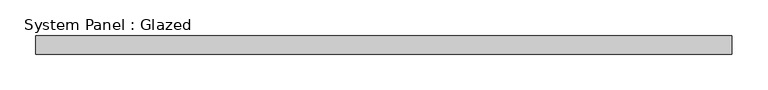
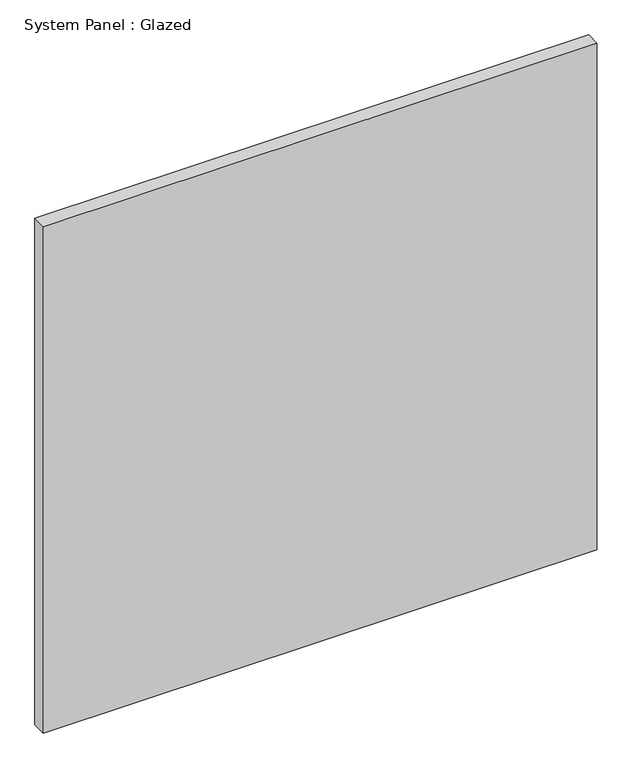
"""IFC4 building model written with IfcOpenShell, lengths in millimetres: plate geometry, System Panel : Glazed."""

from ifc_helpers import new_model, si_unit, origin, origin_with_axes, place, context, project, spatial, polyline, outline, extrude, source, transform, mapped, element, save


def system_panel_glazed_fc95d3d1(model_context):
    return source(origin(), model_context, "Body", "SweptSolid", [
        extrude(outline(polyline([(485.775, 19.05), (-485.775, 19.05), (-485.775, 44.45), (485.775, 44.45), (485.775, 19.05)])), origin_with_axes(), (0.0, 0.0, 1.0), 939.8),
    ])


if __name__ == "__main__":
    model = new_model("IFC4")
    model_context = context("Model", 3, world=origin())
    ifc_project = project(units=[si_unit("LENGTHUNIT", "METRE", prefix="MILLI")], contexts=[model_context])
    site = spatial("IfcSite", under=ifc_project)
    building = spatial("IfcBuilding", under=site)
    placement = place(None, origin())
    system_panel_glazed_shape = system_panel_glazed_fc95d3d1(model_context)
    element("IfcPlate", 1, ObjectType="System Panel : Glazed", at=placement, inside=building, context=model_context, shape_type="MappedRepresentation", body=[
        mapped(system_panel_glazed_shape, transform((0.0, 0.0, 0.0), x_axis=(1.0, 0.0, 0.0), y_axis=(0.0, 1.0, 0.0), z_axis=(0.0, 0.0, 1.0))),
    ])
    save(model, "model.ifc")

# Revit data of these elements
# Type "System Panel : Glazed"
#   Construction Type Id = "GSP4R"
#   Analytic Construction = "1/8 in Pilkington single glazing"
#   Visual Light Transmittance = 0.9
#   Solar Heat Gain Coefficient = 0.86
#   Heat Transfer Coefficient (U) = 1.18115 BTU/(h·ft²·°F)
#   Define Thermal Properties by = 1
# Element 1 (IfcPlate, "System Panel : Glazed")
#   Materials on its faces: "Glass"
# Materials
#   "Glass": class "Glass", colour RGB 0 128 192, transparency 0.75, Description = "Soda Lime Glass", Cost = 0
